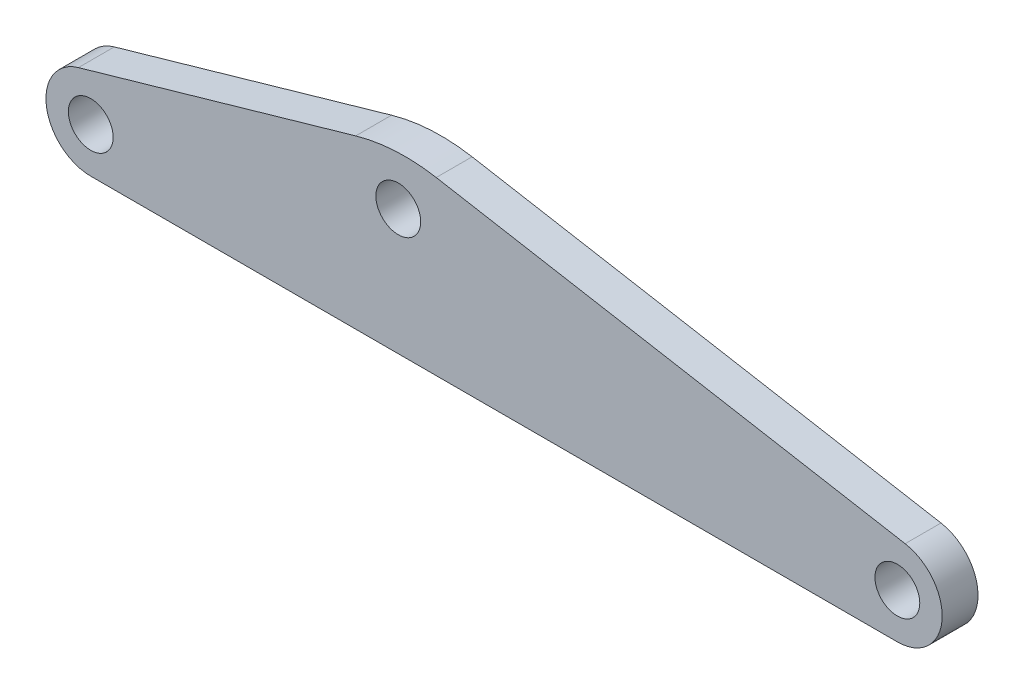
ISO-10303-21;
HEADER;
FILE_DESCRIPTION(('STEP AP214'),'2;1');
FILE_NAME('part.step','',(''),(''),'','','');
FILE_SCHEMA(('AUTOMOTIVE_DESIGN { 1 0 10303 214 1 1 1 1 }'));
ENDSEC;
DATA;
#1=APPLICATION_CONTEXT('core data for automotive mechanical design processes');
#2=APPLICATION_PROTOCOL_DEFINITION('international standard','automotive_design',2000,#1);
#3=PRODUCT_CONTEXT('',#1,'mechanical');
#4=PRODUCT('Part','Part','',(#3));
#5=PRODUCT_RELATED_PRODUCT_CATEGORY('part','',(#4));
#6=PRODUCT_DEFINITION_FORMATION('','',#4);
#7=PRODUCT_DEFINITION_CONTEXT('part definition',#1,'design');
#8=PRODUCT_DEFINITION('design','',#6,#7);
#9=PRODUCT_DEFINITION_SHAPE('','',#8);
#10=(LENGTH_UNIT() NAMED_UNIT(*) SI_UNIT(.MILLI.,.METRE.));
#11=(NAMED_UNIT(*) PLANE_ANGLE_UNIT() SI_UNIT($,.RADIAN.));
#12=(NAMED_UNIT(*) SI_UNIT($,.STERADIAN.) SOLID_ANGLE_UNIT());
#13=UNCERTAINTY_MEASURE_WITH_UNIT(LENGTH_MEASURE(1.E-05),#10,'distance_accuracy_value','');
#14=(GEOMETRIC_REPRESENTATION_CONTEXT(3) GLOBAL_UNCERTAINTY_ASSIGNED_CONTEXT((#13)) GLOBAL_UNIT_ASSIGNED_CONTEXT((#10,
#11,#12)) REPRESENTATION_CONTEXT('',''));
#15=CARTESIAN_POINT('',(0.,0.,0.));
#16=DIRECTION('',(0.,0.,1.));
#17=DIRECTION('',(1.,0.,0.));
#18=AXIS2_PLACEMENT_3D('',#15,#16,#17);
#19=CARTESIAN_POINT('',(52.6017735725068,5.,4.));
#20=DIRECTION('',(0.,0.,1.));
#21=DIRECTION('',(1.,0.,0.));
#22=AXIS2_PLACEMENT_3D('',#19,#20,#21);
#23=PLANE('',#22);
#24=CARTESIAN_POINT('',(-37.3982264274932,4.99999999999999,4.));
#25=DIRECTION('',(0.,0.,1.));
#26=DIRECTION('',(1.,0.,0.));
#27=AXIS2_PLACEMENT_3D('',#24,#25,#26);
#28=CIRCLE('',#27,2.5);
#29=CARTESIAN_POINT('',(-34.8982264274932,4.99999999999999,4.));
#30=VERTEX_POINT('',#29);
#31=EDGE_CURVE('E188',#30,#30,#28,.T.);
#32=ORIENTED_EDGE('',*,*,#31,.F.);
#33=EDGE_LOOP('',(#32));
#34=FACE_BOUND('',#33,.T.);
#35=CARTESIAN_POINT('',(52.6017735725068,5.,4.));
#36=DIRECTION('',(0.,0.,1.));
#37=DIRECTION('',(1.,0.,0.));
#38=AXIS2_PLACEMENT_3D('',#35,#36,#37);
#39=CIRCLE('',#38,5.);
#40=CARTESIAN_POINT('',(52.6017735725068,0.,4.));
#41=VERTEX_POINT('',#40);
#42=CARTESIAN_POINT('',(53.4700144608414,9.92403876506105,4.));
#43=VERTEX_POINT('',#42);
#44=EDGE_CURVE('E133',#41,#43,#39,.T.);
#45=ORIENTED_EDGE('',*,*,#44,.T.);
#46=DIRECTION('',(-0.984807753012209,0.173648177666923,0.));
#47=VECTOR('',#46,1.);
#48=CARTESIAN_POINT('',(1.15029291275593,19.1494172971422,4.));
#49=LINE('',#48,#47);
#50=CARTESIAN_POINT('',(1.15029291275592,19.1494172971422,4.));
#51=VERTEX_POINT('',#50);
#52=EDGE_CURVE('E91',#43,#51,#49,.T.);
#53=ORIENTED_EDGE('',*,*,#52,.T.);
#54=CARTESIAN_POINT('',(-2.32267064058262,-0.54673776310199,4.));
#55=DIRECTION('',(0.,0.,1.));
#56=DIRECTION('',(-1.,0.,0.));
#57=AXIS2_PLACEMENT_3D('',#54,#55,#56);
#58=CIRCLE('',#57,20.);
#59=CARTESIAN_POINT('',(-7.83541775692254,18.6784961556644,4.));
#60=VERTEX_POINT('',#59);
#61=EDGE_CURVE('E106',#51,#60,#58,.T.);
#62=ORIENTED_EDGE('',*,*,#61,.T.);
#63=DIRECTION('',(-0.961261695938321,-0.275637355816993,0.));
#64=VECTOR('',#63,1.);
#65=CARTESIAN_POINT('',(-38.7764132065782,9.80630847969159,4.));
#66=LINE('',#65,#64);
#67=CARTESIAN_POINT('',(-38.7764132065782,9.80630847969159,4.));
#68=VERTEX_POINT('',#67);
#69=EDGE_CURVE('E99',#60,#68,#66,.T.);
#70=ORIENTED_EDGE('',*,*,#69,.T.);
#71=CARTESIAN_POINT('',(-37.3982264274932,4.99999999999999,4.));
#72=DIRECTION('',(0.,0.,1.));
#73=DIRECTION('',(1.,0.,0.));
#74=AXIS2_PLACEMENT_3D('',#71,#72,#73);
#75=CIRCLE('',#74,5.);
#76=CARTESIAN_POINT('',(-37.3982264274932,0.,4.));
#77=VERTEX_POINT('',#76);
#78=EDGE_CURVE('E102',#68,#77,#75,.T.);
#79=ORIENTED_EDGE('',*,*,#78,.T.);
#80=DIRECTION('',(1.,0.,0.));
#81=VECTOR('',#80,1.);
#82=CARTESIAN_POINT('',(52.6017735725068,0.,4.));
#83=LINE('',#82,#81);
#84=EDGE_CURVE('E57',#77,#41,#83,.T.);
#85=ORIENTED_EDGE('',*,*,#84,.T.);
#86=EDGE_LOOP('',(#45,#53,#62,#70,#79,#85));
#87=FACE_BOUND('',#86,.T.);
#88=CARTESIAN_POINT('',(-3.08503286255954,14.,4.));
#89=DIRECTION('',(0.,0.,1.));
#90=DIRECTION('',(1.,0.,0.));
#91=AXIS2_PLACEMENT_3D('',#88,#89,#90);
#92=CIRCLE('',#91,2.5);
#93=CARTESIAN_POINT('',(-0.585032862559536,14.,4.));
#94=VERTEX_POINT('',#93);
#95=EDGE_CURVE('E126',#94,#94,#92,.T.);
#96=ORIENTED_EDGE('',*,*,#95,.F.);
#97=EDGE_LOOP('',(#96));
#98=FACE_BOUND('',#97,.T.);
#99=CARTESIAN_POINT('',(52.6017735725068,5.,4.));
#100=DIRECTION('',(0.,0.,1.));
#101=DIRECTION('',(1.,0.,0.));
#102=AXIS2_PLACEMENT_3D('',#99,#100,#101);
#103=CIRCLE('',#102,2.5);
#104=CARTESIAN_POINT('',(55.1017735725068,5.,4.));
#105=VERTEX_POINT('',#104);
#106=EDGE_CURVE('E182',#105,#105,#103,.T.);
#107=ORIENTED_EDGE('',*,*,#106,.F.);
#108=EDGE_LOOP('',(#107));
#109=FACE_BOUND('',#108,.T.);
#110=ADVANCED_FACE('F39',(#34,#87,#98,#109),#23,.T.);
#111=CARTESIAN_POINT('',(52.6017735725068,5.,0.));
#112=DIRECTION('',(0.,0.,1.));
#113=DIRECTION('',(1.,0.,0.));
#114=AXIS2_PLACEMENT_3D('',#111,#112,#113);
#115=PLANE('',#114);
#116=CARTESIAN_POINT('',(52.6017735725068,5.,0.));
#117=DIRECTION('',(0.,0.,1.));
#118=DIRECTION('',(1.,0.,0.));
#119=AXIS2_PLACEMENT_3D('',#116,#117,#118);
#120=CIRCLE('',#119,5.);
#121=CARTESIAN_POINT('',(52.6017735725068,0.,0.));
#122=VERTEX_POINT('',#121);
#123=CARTESIAN_POINT('',(53.4700144608414,9.92403876506105,0.));
#124=VERTEX_POINT('',#123);
#125=EDGE_CURVE('E121',#122,#124,#120,.T.);
#126=ORIENTED_EDGE('',*,*,#125,.F.);
#127=DIRECTION('',(1.,0.,0.));
#128=VECTOR('',#127,1.);
#129=CARTESIAN_POINT('',(52.6017735725068,0.,0.));
#130=LINE('',#129,#128);
#131=CARTESIAN_POINT('',(-37.3982264274932,0.,0.));
#132=VERTEX_POINT('',#131);
#133=EDGE_CURVE('E83',#132,#122,#130,.T.);
#134=ORIENTED_EDGE('',*,*,#133,.F.);
#135=CARTESIAN_POINT('',(-37.3982264274932,4.99999999999999,0.));
#136=DIRECTION('',(0.,0.,1.));
#137=DIRECTION('',(1.,0.,0.));
#138=AXIS2_PLACEMENT_3D('',#135,#136,#137);
#139=CIRCLE('',#138,5.);
#140=CARTESIAN_POINT('',(-38.7764132065782,9.80630847969159,0.));
#141=VERTEX_POINT('',#140);
#142=EDGE_CURVE('E76',#141,#132,#139,.T.);
#143=ORIENTED_EDGE('',*,*,#142,.F.);
#144=DIRECTION('',(-0.961261695938321,-0.275637355816993,0.));
#145=VECTOR('',#144,1.);
#146=CARTESIAN_POINT('',(-38.7764132065782,9.80630847969159,0.));
#147=LINE('',#146,#145);
#148=CARTESIAN_POINT('',(-7.83541775692254,18.6784961556644,0.));
#149=VERTEX_POINT('',#148);
#150=EDGE_CURVE('E111',#149,#141,#147,.T.);
#151=ORIENTED_EDGE('',*,*,#150,.F.);
#152=CARTESIAN_POINT('',(-2.32267064058262,-0.54673776310199,0.));
#153=DIRECTION('',(0.,0.,1.));
#154=DIRECTION('',(-1.,0.,0.));
#155=AXIS2_PLACEMENT_3D('',#152,#153,#154);
#156=CIRCLE('',#155,20.);
#157=CARTESIAN_POINT('',(1.15029291275592,19.1494172971422,0.));
#158=VERTEX_POINT('',#157);
#159=EDGE_CURVE('E128',#158,#149,#156,.T.);
#160=ORIENTED_EDGE('',*,*,#159,.F.);
#161=DIRECTION('',(-0.984807753012209,0.173648177666923,0.));
#162=VECTOR('',#161,1.);
#163=CARTESIAN_POINT('',(1.15029291275593,19.1494172971422,0.));
#164=LINE('',#163,#162);
#165=EDGE_CURVE('E130',#124,#158,#164,.T.);
#166=ORIENTED_EDGE('',*,*,#165,.F.);
#167=EDGE_LOOP('',(#126,#134,#143,#151,#160,#166));
#168=FACE_BOUND('',#167,.T.);
#169=CARTESIAN_POINT('',(-3.08503286255954,14.,0.));
#170=DIRECTION('',(0.,0.,1.));
#171=DIRECTION('',(1.,0.,0.));
#172=AXIS2_PLACEMENT_3D('',#169,#170,#171);
#173=CIRCLE('',#172,2.5);
#174=CARTESIAN_POINT('',(-0.585032862559536,14.,0.));
#175=VERTEX_POINT('',#174);
#176=EDGE_CURVE('E195',#175,#175,#173,.T.);
#177=ORIENTED_EDGE('',*,*,#176,.T.);
#178=EDGE_LOOP('',(#177));
#179=FACE_BOUND('',#178,.T.);
#180=CARTESIAN_POINT('',(-37.3982264274932,4.99999999999999,0.));
#181=DIRECTION('',(0.,0.,1.));
#182=DIRECTION('',(1.,0.,0.));
#183=AXIS2_PLACEMENT_3D('',#180,#181,#182);
#184=CIRCLE('',#183,2.5);
#185=CARTESIAN_POINT('',(-34.8982264274932,4.99999999999999,0.));
#186=VERTEX_POINT('',#185);
#187=EDGE_CURVE('E190',#186,#186,#184,.T.);
#188=ORIENTED_EDGE('',*,*,#187,.T.);
#189=EDGE_LOOP('',(#188));
#190=FACE_BOUND('',#189,.T.);
#191=CARTESIAN_POINT('',(52.6017735725068,5.,0.));
#192=DIRECTION('',(0.,0.,1.));
#193=DIRECTION('',(1.,0.,0.));
#194=AXIS2_PLACEMENT_3D('',#191,#192,#193);
#195=CIRCLE('',#194,2.5);
#196=CARTESIAN_POINT('',(55.1017735725068,5.,0.));
#197=VERTEX_POINT('',#196);
#198=EDGE_CURVE('E184',#197,#197,#195,.T.);
#199=ORIENTED_EDGE('',*,*,#198,.T.);
#200=EDGE_LOOP('',(#199));
#201=FACE_BOUND('',#200,.T.);
#202=ADVANCED_FACE('F145',(#168,#179,#190,#201),#115,.F.);
#203=CARTESIAN_POINT('',(52.6017735725068,5.,4.));
#204=DIRECTION('',(0.,0.,-1.));
#205=DIRECTION('',(-1.,0.,0.));
#206=AXIS2_PLACEMENT_3D('',#203,#204,#205);
#207=CYLINDRICAL_SURFACE('',#206,5.);
#208=ORIENTED_EDGE('',*,*,#125,.T.);
#209=DIRECTION('',(0.,0.,-1.));
#210=VECTOR('',#209,1.);
#211=CARTESIAN_POINT('',(53.4700144608414,9.92403876506105,4.));
#212=LINE('',#211,#210);
#213=EDGE_CURVE('E11',#43,#124,#212,.T.);
#214=ORIENTED_EDGE('',*,*,#213,.F.);
#215=ORIENTED_EDGE('',*,*,#44,.F.);
#216=DIRECTION('',(0.,0.,-1.));
#217=VECTOR('',#216,1.);
#218=CARTESIAN_POINT('',(52.6017735725068,0.,4.));
#219=LINE('',#218,#217);
#220=EDGE_CURVE('E118',#41,#122,#219,.T.);
#221=ORIENTED_EDGE('',*,*,#220,.T.);
#222=EDGE_LOOP('',(#208,#214,#215,#221));
#223=FACE_BOUND('',#222,.T.);
#224=ADVANCED_FACE('F41',(#223),#207,.T.);
#225=CARTESIAN_POINT('',(1.15029291275593,19.1494172971422,4.));
#226=DIRECTION('',(-0.173648177666923,-0.984807753012209,0.));
#227=DIRECTION('',(0.984807753012209,-0.173648177666923,0.));
#228=AXIS2_PLACEMENT_3D('',#225,#226,#227);
#229=PLANE('',#228);
#230=ORIENTED_EDGE('',*,*,#165,.T.);
#231=DIRECTION('',(0.,0.,-1.));
#232=VECTOR('',#231,1.);
#233=CARTESIAN_POINT('',(1.15029291275592,19.1494172971422,4.));
#234=LINE('',#233,#232);
#235=EDGE_CURVE('E48',#51,#158,#234,.T.);
#236=ORIENTED_EDGE('',*,*,#235,.F.);
#237=ORIENTED_EDGE('',*,*,#52,.F.);
#238=ORIENTED_EDGE('',*,*,#213,.T.);
#239=EDGE_LOOP('',(#230,#236,#237,#238));
#240=FACE_BOUND('',#239,.T.);
#241=ADVANCED_FACE('F247',(#240),#229,.F.);
#242=CARTESIAN_POINT('',(-2.32267064058262,-0.54673776310199,4.));
#243=DIRECTION('',(0.,0.,-1.));
#244=DIRECTION('',(-1.,0.,0.));
#245=AXIS2_PLACEMENT_3D('',#242,#243,#244);
#246=CYLINDRICAL_SURFACE('',#245,20.);
#247=ORIENTED_EDGE('',*,*,#159,.T.);
#248=DIRECTION('',(0.,0.,-1.));
#249=VECTOR('',#248,1.);
#250=CARTESIAN_POINT('',(-7.83541775692254,18.6784961556644,4.));
#251=LINE('',#250,#249);
#252=EDGE_CURVE('E113',#60,#149,#251,.T.);
#253=ORIENTED_EDGE('',*,*,#252,.F.);
#254=ORIENTED_EDGE('',*,*,#61,.F.);
#255=ORIENTED_EDGE('',*,*,#235,.T.);
#256=EDGE_LOOP('',(#247,#253,#254,#255));
#257=FACE_BOUND('',#256,.T.);
#258=ADVANCED_FACE('F143',(#257),#246,.T.);
#259=CARTESIAN_POINT('',(-38.7764132065782,9.80630847969159,4.));
#260=DIRECTION('',(0.275637355816993,-0.961261695938321,0.));
#261=DIRECTION('',(0.961261695938321,0.275637355816993,0.));
#262=AXIS2_PLACEMENT_3D('',#259,#260,#261);
#263=PLANE('',#262);
#264=ORIENTED_EDGE('',*,*,#150,.T.);
#265=DIRECTION('',(0.,0.,-1.));
#266=VECTOR('',#265,1.);
#267=CARTESIAN_POINT('',(-38.7764132065782,9.80630847969159,4.));
#268=LINE('',#267,#266);
#269=EDGE_CURVE('E112',#68,#141,#268,.T.);
#270=ORIENTED_EDGE('',*,*,#269,.F.);
#271=ORIENTED_EDGE('',*,*,#69,.F.);
#272=ORIENTED_EDGE('',*,*,#252,.T.);
#273=EDGE_LOOP('',(#264,#270,#271,#272));
#274=FACE_BOUND('',#273,.T.);
#275=ADVANCED_FACE('F115',(#274),#263,.F.);
#276=CARTESIAN_POINT('',(-37.3982264274932,4.99999999999999,4.));
#277=DIRECTION('',(0.,0.,-1.));
#278=DIRECTION('',(-1.,0.,0.));
#279=AXIS2_PLACEMENT_3D('',#276,#277,#278);
#280=CYLINDRICAL_SURFACE('',#279,5.);
#281=ORIENTED_EDGE('',*,*,#142,.T.);
#282=DIRECTION('',(0.,0.,-1.));
#283=VECTOR('',#282,1.);
#284=CARTESIAN_POINT('',(-37.3982264274932,0.,4.));
#285=LINE('',#284,#283);
#286=EDGE_CURVE('E117',#77,#132,#285,.T.);
#287=ORIENTED_EDGE('',*,*,#286,.F.);
#288=ORIENTED_EDGE('',*,*,#78,.F.);
#289=ORIENTED_EDGE('',*,*,#269,.T.);
#290=EDGE_LOOP('',(#281,#287,#288,#289));
#291=FACE_BOUND('',#290,.T.);
#292=ADVANCED_FACE('F119',(#291),#280,.T.);
#293=CARTESIAN_POINT('',(52.6017735725068,0.,4.));
#294=DIRECTION('',(0.,1.,0.));
#295=DIRECTION('',(-1.,0.,0.));
#296=AXIS2_PLACEMENT_3D('',#293,#294,#295);
#297=PLANE('',#296);
#298=ORIENTED_EDGE('',*,*,#133,.T.);
#299=ORIENTED_EDGE('',*,*,#220,.F.);
#300=ORIENTED_EDGE('',*,*,#84,.F.);
#301=ORIENTED_EDGE('',*,*,#286,.T.);
#302=EDGE_LOOP('',(#298,#299,#300,#301));
#303=FACE_BOUND('',#302,.T.);
#304=ADVANCED_FACE('F149',(#303),#297,.F.);
#305=CARTESIAN_POINT('',(-3.08503286255954,14.,4.));
#306=DIRECTION('',(0.,0.,-1.));
#307=DIRECTION('',(-1.,0.,0.));
#308=AXIS2_PLACEMENT_3D('',#305,#306,#307);
#309=CYLINDRICAL_SURFACE('',#308,2.5);
#310=ORIENTED_EDGE('',*,*,#95,.T.);
#311=EDGE_LOOP('',(#310));
#312=FACE_BOUND('',#311,.T.);
#313=ORIENTED_EDGE('',*,*,#176,.F.);
#314=EDGE_LOOP('',(#313));
#315=FACE_BOUND('',#314,.T.);
#316=ADVANCED_FACE('F151',(#312,#315),#309,.F.);
#317=CARTESIAN_POINT('',(-37.3982264274932,4.99999999999999,4.));
#318=DIRECTION('',(0.,0.,-1.));
#319=DIRECTION('',(-1.,0.,0.));
#320=AXIS2_PLACEMENT_3D('',#317,#318,#319);
#321=CYLINDRICAL_SURFACE('',#320,2.5);
#322=ORIENTED_EDGE('',*,*,#31,.T.);
#323=EDGE_LOOP('',(#322));
#324=FACE_BOUND('',#323,.T.);
#325=ORIENTED_EDGE('',*,*,#187,.F.);
#326=EDGE_LOOP('',(#325));
#327=FACE_BOUND('',#326,.T.);
#328=ADVANCED_FACE('F160',(#324,#327),#321,.F.);
#329=CARTESIAN_POINT('',(52.6017735725068,5.,4.));
#330=DIRECTION('',(0.,0.,-1.));
#331=DIRECTION('',(-1.,0.,0.));
#332=AXIS2_PLACEMENT_3D('',#329,#330,#331);
#333=CYLINDRICAL_SURFACE('',#332,2.5);
#334=ORIENTED_EDGE('',*,*,#106,.T.);
#335=EDGE_LOOP('',(#334));
#336=FACE_BOUND('',#335,.T.);
#337=ORIENTED_EDGE('',*,*,#198,.F.);
#338=EDGE_LOOP('',(#337));
#339=FACE_BOUND('',#338,.T.);
#340=ADVANCED_FACE('F175',(#336,#339),#333,.F.);
#341=CLOSED_SHELL('',(#110,#202,#224,#241,#258,#275,#292,#304,#316,#328,#340));
#342=MANIFOLD_SOLID_BREP('B2',#341);
#343=ADVANCED_BREP_SHAPE_REPRESENTATION('',(#18,#342),#14);
#344=SHAPE_DEFINITION_REPRESENTATION(#9,#343);
ENDSEC;
END-ISO-10303-21;
